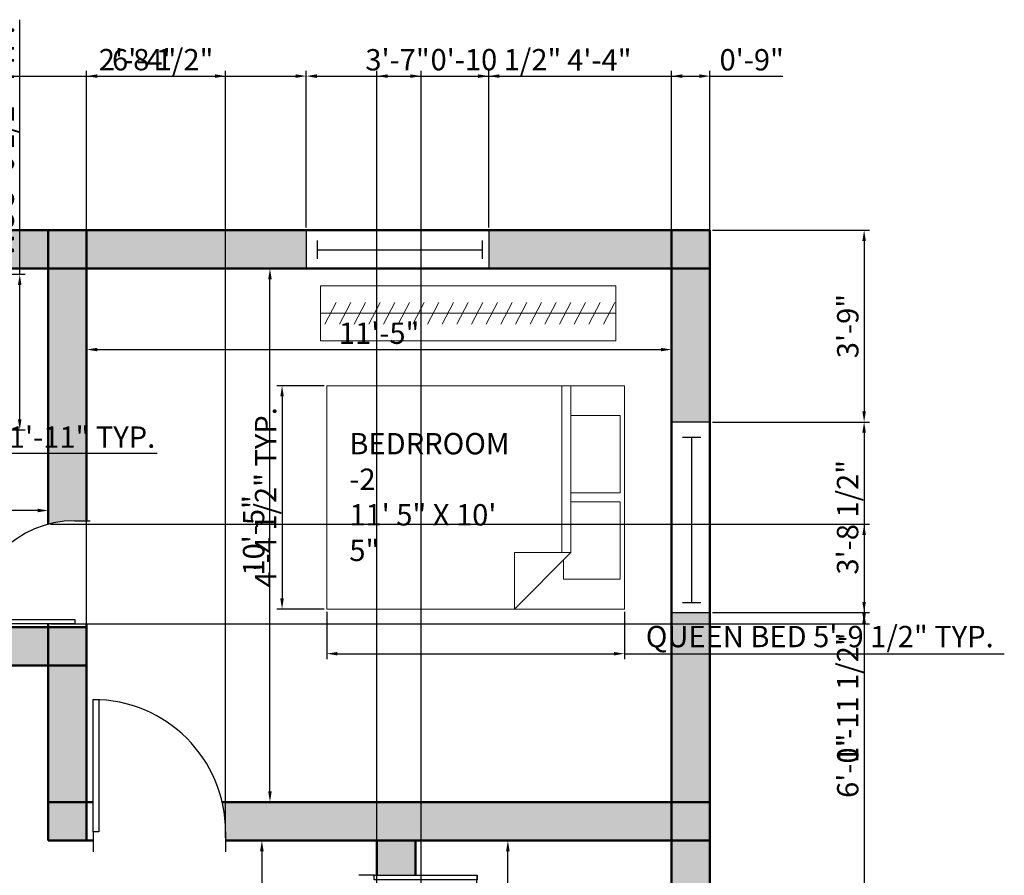
# Model space of a CAD drawing. Units: millimetres. Extents: x 2784 to 3697, y 603 to 1406.
# Tile 7 of 10: x 3013 to 3244, y 1205 to 1406. Entities that reach past the tile are written whole.
import ezdxf

# ---------------------------------------------------------------- set-up
doc = ezdxf.new("R2010")
doc.units = ezdxf.units.MM
for name, color, linetype, lineweight in [('A-ANNO-DIMS', 140, 'Continuous', 18), ('A-AREA-IDEN', 150, 'Continuous', 25), ('A-DOOR', 10, 'Continuous', 25), ('A-FURN', 80, 'Continuous', 18), ('A-GLAZ', 30, 'Continuous', 25), ('A-WALL', 2, 'Continuous', 50), ('A-WALL-PATT', 8, 'Continuous', 13)]:
    doc.layers.add(name, color=color, linetype=linetype, lineweight=lineweight)
doc.styles.get("Standard").update_dxf_attribs({"font": 'arial.ttf'})
doc.dimstyles.new('ISO-25', dxfattribs={"dimtxt": 5, "dimasz": 2.5, "dimexe": 1.25, "dimexo": 0.625, "dimtad": 1, "dimdec": 0, "dimlunit": 3, "dimtxsty": 'Standard', "dimcen": 2.5, "dimadec": 0, "dimazin": 0, "dimtfac": 1, "dimtdec": 0, "dimtmove": 0, "dimatfit": 3, "dimfxl": 1, "dimarcsym": 0})

# ---------------------------------------------------------------- blocks, each defined once
blk = doc.blocks.new('*U2')
for p, q in [((0, 0), (0, -6)), ((40, 0), (40, -6))]:
    blk.add_line(p, q)
blk.add_lwpolyline([(0, 0), (0, 40), (1.75, 40), (1.75, 0)], close=True)
blk.add_arc((0, 0), 40, 0, 90)
blk = doc.blocks.new('*U4')
for p, q in [((0, 4), (0, 0)), ((36, 4), (36, 0)), ((0, 2), (36, 2))]:
    blk.add_line(p, q)
blk = doc.blocks.new('Bed - Queen')
for p, q in [((0, -80.00003), (0, 0)), ((0, 0), (59.99999, 0)), ((59.99999, 0), (59.99999, -80.00003)), ((7.99999, -1.2), (28.79998, -1.2)), ((7.99999, -14.4), (7.99999, -1.2)), ((28.79998, -1.2), (28.79998, -14.4)), ((31.19999, -1.2), (51.99999, -1.2)), ((31.19999, -14.4), (31.19999, -1.2)), ((51.99999, -1.2), (51.99999, -16.4)), ((0, -14.4), (44.8, -14.4)), ((59.99999, -29.6), (44.8, -14.4)), ((44.8, -14.4), (44.8, -29.6)), ((44.8, -16.8), (0, -16.8)), ((51.99999, -16.4), (46.79936, -16.4)), ((44.8, -29.6), (59.99999, -29.6)), ((59.99999, -80.00003), (0, -80.00003))]:
    blk.add_line(p, q)
blk = doc.blocks.new('*D18')
at = {"layer": 'A-ANNO-DIMS', "color": 0, "lineweight": -2, "transparency": 16777216}
for p, q in [((2971.91, 1291.46), (2971.91, 1289.3)), ((3019.91, 1291.46), (3019.91, 1289.3)), ((3017.41, 1290.55), (2974.41, 1290.55))]:
    blk.add_line(p, q, dxfattribs=at)
at = {"layer": 'A-ANNO-DIMS', "color": 0, "transparency": 16777216}
for points in [[(2974.41, 1290.97), (2974.41, 1290.13), (2971.91, 1290.55)], [(3017.41, 1290.97), (3017.41, 1290.13), (3019.91, 1290.55)]]:
    blk.add_solid(points, dxfattribs=at)
at = {"layer": 'Defpoints', "color": 0, "transparency": 16777216}
for p in [(2971.91, 1292.08), (3019.91, 1292.08), (2971.91, 1290.55)]:
    blk.add_point(p, dxfattribs=at)
at = {"layer": 'A-ANNO-DIMS', "color": 0, "transparency": 16777216, "insert": (2995.91, 1293.67), "char_height": 5, "attachment_point": 5}
blk.add_mtext("4'", dxfattribs=at)
blk = doc.blocks.new('*D19')
at = {"layer": 'A-ANNO-DIMS', "color": 0, "lineweight": -2, "transparency": 16777216}
for p, q in [((3072.89, 1347.23), (3070.59, 1347.23)), ((3071.84, 1224.73), (3071.84, 1344.73)), ((3072.89, 1222.23), (3070.59, 1222.23))]:
    blk.add_line(p, q, dxfattribs=at)
at = {"layer": 'A-ANNO-DIMS', "color": 0, "transparency": 16777216}
for points in [[(3071.43, 1344.73), (3072.26, 1344.73), (3071.84, 1347.23)], [(3071.43, 1224.73), (3072.26, 1224.73), (3071.84, 1222.23)]]:
    blk.add_solid(points, dxfattribs=at)
at = {"layer": 'Defpoints', "color": 0, "transparency": 16777216}
for p in [(3071.84, 1347.23), (3073.51, 1347.23), (3073.51, 1222.23)]:
    blk.add_point(p, dxfattribs=at)
at = {"layer": 'A-ANNO-DIMS', "color": 0, "transparency": 16777216, "insert": (3068.66, 1284.73), "char_height": 5, "attachment_point": 5, "rotation": 90}
blk.add_mtext('10\'-5"', dxfattribs=at)
blk = doc.blocks.new('*D20')
at = {"layer": 'A-ANNO-DIMS', "color": 0, "lineweight": -2, "transparency": 16777216}
for p, q in [((3028.91, 1322.82), (3028.91, 1329.51)), ((3165.91, 1328.88), (3165.91, 1329.51)), ((3031.41, 1328.26), (3163.41, 1328.26))]:
    blk.add_line(p, q, dxfattribs=at)
at = {"layer": 'A-ANNO-DIMS', "color": 0, "transparency": 16777216}
for points in [[(3031.41, 1328.67), (3031.41, 1327.84), (3028.91, 1328.26)], [(3163.41, 1328.67), (3163.41, 1327.84), (3165.91, 1328.26)]]:
    blk.add_solid(points, dxfattribs=at)
at = {"layer": 'Defpoints', "color": 0, "transparency": 16777216}
for p in [(3165.91, 1328.26), (3165.91, 1328.26), (3028.91, 1322.19)]:
    blk.add_point(p, dxfattribs=at)
at = {"layer": 'A-ANNO-DIMS', "color": 0, "transparency": 16777216, "insert": (3097.41, 1331.44), "char_height": 5, "attachment_point": 5}
blk.add_mtext('11\'-5"', dxfattribs=at)
blk = doc.blocks.new('*D24')
at = {"layer": 'A-ANNO-DIMS', "color": 0, "lineweight": -2, "transparency": 16777216}
for p, q in [((3124.34, 1213.23), (3128.82, 1213.23)), ((3127.57, 1150.73), (3127.57, 1210.73)), ((3124.34, 1148.23), (3128.82, 1148.23))]:
    blk.add_line(p, q, dxfattribs=at)
at = {"layer": 'A-ANNO-DIMS', "color": 0, "transparency": 16777216}
for points in [[(3127.15, 1210.73), (3127.98, 1210.73), (3127.57, 1213.23)], [(3127.15, 1150.73), (3127.98, 1150.73), (3127.57, 1148.23)]]:
    blk.add_solid(points, dxfattribs=at)
at = {"layer": 'Defpoints', "color": 0, "transparency": 16777216}
for p in [(3123.72, 1213.23), (3127.57, 1213.23), (3123.72, 1148.23)]:
    blk.add_point(p, dxfattribs=at)
at = {"layer": 'A-ANNO-DIMS', "color": 0, "transparency": 16777216, "insert": (3124.4, 1180.73), "char_height": 5, "attachment_point": 5, "rotation": 90}
blk.add_mtext('5\'-5"', dxfattribs=at)
blk = doc.blocks.new('*D37')
at = {"layer": 'A-ANNO-DIMS', "color": 0, "lineweight": -2, "transparency": 16777216}
for p, q in [((3069.6, 1213.23), (3068.7, 1213.23)), ((3069.95, 1210.73), (3069.95, 1081.73)), ((3069.6, 1079.23), (3068.7, 1079.23))]:
    blk.add_line(p, q, dxfattribs=at)
at = {"layer": 'A-ANNO-DIMS', "color": 0, "transparency": 16777216}
for points in [[(3069.53, 1210.73), (3070.37, 1210.73), (3069.95, 1213.23)], [(3069.53, 1081.73), (3070.37, 1081.73), (3069.95, 1079.23)]]:
    blk.add_solid(points, dxfattribs=at)
at = {"layer": 'Defpoints', "color": 0, "transparency": 16777216}
for p in [(3070.22, 1213.23), (3069.95, 1079.23), (3070.22, 1079.23)]:
    blk.add_point(p, dxfattribs=at)
at = {"layer": 'A-ANNO-DIMS', "color": 0, "transparency": 16777216, "insert": (3066.81, 1146.23), "char_height": 5, "attachment_point": 5, "rotation": 90}
blk.add_mtext('11\'-2"', dxfattribs=at)
blk = doc.blocks.new('*D60')
at = {"layer": 'A-ANNO-DIMS', "color": 0, "lineweight": -2, "transparency": 16777216}
for p, q in [((3085.15, 1266.84), (3085.15, 1255.75)), ((3154.89, 1266.84), (3154.89, 1255.75)), ((3087.65, 1257), (3152.39, 1257)), ((3154.89, 1257), (3243.84, 1257))]:
    blk.add_line(p, q, dxfattribs=at)
at = {"layer": 'A-ANNO-DIMS', "color": 0, "transparency": 16777216}
for points in [[(3087.65, 1257.42), (3087.65, 1256.59), (3085.15, 1257)], [(3152.39, 1257.42), (3152.39, 1256.59), (3154.89, 1257)]]:
    blk.add_solid(points, dxfattribs=at)
at = {"layer": 'Defpoints', "color": 0, "transparency": 16777216}
for p in [(3085.15, 1267.47), (3154.89, 1267.47), (3154.89, 1257)]:
    blk.add_point(p, dxfattribs=at)
at = {"layer": 'A-ANNO-DIMS', "color": 0, "transparency": 16777216, "insert": (3200.62, 1260.37), "char_height": 5, "attachment_point": 5}
blk.add_mtext('QUEEN BED 5\'-9 1/2" TYP.', dxfattribs=at)
blk = doc.blocks.new('*D61')
at = {"layer": 'A-ANNO-DIMS', "color": 0, "lineweight": -2, "transparency": 16777216}
for p, q in [((3084.52, 1319.77), (3073.43, 1319.77)), ((3074.68, 1317.27), (3074.68, 1269.97)), ((3084.52, 1267.47), (3073.43, 1267.47))]:
    blk.add_line(p, q, dxfattribs=at)
at = {"layer": 'A-ANNO-DIMS', "color": 0, "transparency": 16777216}
for points in [[(3074.27, 1317.27), (3075.1, 1317.27), (3074.68, 1319.77)], [(3074.27, 1269.97), (3075.1, 1269.97), (3074.68, 1267.47)]]:
    blk.add_solid(points, dxfattribs=at)
at = {"layer": 'Defpoints', "color": 0, "transparency": 16777216}
for p in [(3085.15, 1319.77), (3074.68, 1267.47), (3085.15, 1267.47)]:
    blk.add_point(p, dxfattribs=at)
at = {"layer": 'A-ANNO-DIMS', "color": 0, "transparency": 16777216, "insert": (3071.47, 1293.62), "char_height": 5, "attachment_point": 5, "rotation": 90}
blk.add_mtext('4\'-4 1/2" TYP.', dxfattribs=at)
blk = doc.blocks.new('*D72')
at = {"layer": 'A-ANNO-DIMS', "color": 0, "lineweight": -2, "transparency": 16777216}
for p, q in [((3013.24, 1345.89), (3013.24, 1405.55)), ((3008.39, 1345.89), (3014.49, 1345.89)), ((3013.24, 1311.94), (3013.24, 1343.39)), ((3008.39, 1309.44), (3014.49, 1309.44))]:
    blk.add_line(p, q, dxfattribs=at)
at = {"layer": 'A-ANNO-DIMS', "color": 0, "transparency": 16777216}
for points in [[(3012.82, 1343.39), (3013.65, 1343.39), (3013.24, 1345.89)], [(3012.82, 1311.94), (3013.65, 1311.94), (3013.24, 1309.44)]]:
    blk.add_solid(points, dxfattribs=at)
at = {"layer": 'Defpoints', "color": 0, "transparency": 16777216}
for p in [(3007.77, 1345.89), (3013.24, 1345.89), (3007.77, 1309.44)]:
    blk.add_point(p, dxfattribs=at)
at = {"layer": 'A-ANNO-DIMS', "color": 0, "transparency": 16777216, "insert": (3010.03, 1376.97), "char_height": 5, "attachment_point": 5, "rotation": 90}
blk.add_mtext('WC 3\'-0 1/2" TYP.', dxfattribs=at)
blk = doc.blocks.new('*D73')
at = {"layer": 'A-ANNO-DIMS', "color": 0, "lineweight": -2, "transparency": 16777216}
for p, q in [((2984.6, 1308.81), (2984.6, 1302.72)), ((3007.77, 1308.81), (3007.77, 1302.72)), ((2987.1, 1303.97), (3005.27, 1303.97)), ((3007.77, 1303.97), (3045.41, 1303.97))]:
    blk.add_line(p, q, dxfattribs=at)
at = {"layer": 'A-ANNO-DIMS', "color": 0, "transparency": 16777216}
for points in [[(2987.1, 1304.38), (2987.1, 1303.55), (2984.6, 1303.97)], [(3005.27, 1304.38), (3005.27, 1303.55), (3007.77, 1303.97)]]:
    blk.add_solid(points, dxfattribs=at)
at = {"layer": 'Defpoints', "color": 0, "transparency": 16777216}
for p in [(2984.6, 1309.44), (3007.77, 1309.44), (3007.77, 1303.97)]:
    blk.add_point(p, dxfattribs=at)
at = {"layer": 'A-ANNO-DIMS', "color": 0, "transparency": 16777216, "insert": (3027.84, 1307.1), "char_height": 5, "attachment_point": 5}
blk.add_mtext('1\'-11" TYP.', dxfattribs=at)
blk = doc.blocks.new('*D80')
at = {"layer": 'A-ANNO-DIMS', "color": 0, "lineweight": -2, "transparency": 16777216}
for p, q in [((3004.44, 1356.86), (3004.44, 1393.58)), ((3080.34, 1356.86), (3080.34, 1393.58)), ((3006.94, 1392.33), (3077.84, 1392.33))]:
    blk.add_line(p, q, dxfattribs=at)
at = {"layer": 'A-ANNO-DIMS', "color": 0, "transparency": 16777216}
for points in [[(3006.94, 1392.75), (3006.94, 1391.91), (3004.44, 1392.33)], [(3077.84, 1392.75), (3077.84, 1391.91), (3080.34, 1392.33)]]:
    blk.add_solid(points, dxfattribs=at)
at = {"layer": 'Defpoints', "color": 0, "transparency": 16777216}
for p in [(3080.34, 1392.33), (3004.44, 1356.23), (3080.34, 1356.23)]:
    blk.add_point(p, dxfattribs=at)
at = {"layer": 'A-ANNO-DIMS', "color": 0, "transparency": 16777216, "insert": (3042.39, 1395.51), "char_height": 5, "attachment_point": 5}
blk.add_mtext('6\'-4"', dxfattribs=at)
blk = doc.blocks.new('*D81')
at = {"layer": 'A-ANNO-DIMS', "color": 0, "lineweight": -2, "transparency": 16777216}
for p, q in [((3080.34, 1356.86), (3080.34, 1393.58)), ((3123.1, 1356.86), (3123.1, 1393.58)), ((3082.84, 1392.33), (3120.6, 1392.33))]:
    blk.add_line(p, q, dxfattribs=at)
at = {"layer": 'A-ANNO-DIMS', "color": 0, "transparency": 16777216}
for points in [[(3082.84, 1392.75), (3082.84, 1391.91), (3080.34, 1392.33)], [(3120.6, 1392.75), (3120.6, 1391.91), (3123.1, 1392.33)]]:
    blk.add_solid(points, dxfattribs=at)
at = {"layer": 'Defpoints', "color": 0, "transparency": 16777216}
for p in [(3123.1, 1392.33), (3080.34, 1356.23), (3123.1, 1356.23)]:
    blk.add_point(p, dxfattribs=at)
at = {"layer": 'A-ANNO-DIMS', "color": 0, "transparency": 16777216, "insert": (3101.72, 1395.51), "char_height": 5, "attachment_point": 5}
blk.add_mtext('3\'-7"', dxfattribs=at)
blk = doc.blocks.new('*D82')
at = {"layer": 'A-ANNO-DIMS', "color": 0, "lineweight": -2, "transparency": 16777216}
for p, q in [((3123.1, 1356.86), (3123.1, 1393.58)), ((3174.91, 1356.86), (3174.91, 1393.58)), ((3125.6, 1392.33), (3172.41, 1392.33))]:
    blk.add_line(p, q, dxfattribs=at)
at = {"layer": 'A-ANNO-DIMS', "color": 0, "transparency": 16777216}
for points in [[(3125.6, 1392.75), (3125.6, 1391.91), (3123.1, 1392.33)], [(3172.41, 1392.75), (3172.41, 1391.91), (3174.91, 1392.33)]]:
    blk.add_solid(points, dxfattribs=at)
at = {"layer": 'Defpoints', "color": 0, "transparency": 16777216}
for p in [(3174.91, 1392.33), (3123.1, 1356.23), (3174.91, 1356.23)]:
    blk.add_point(p, dxfattribs=at)
at = {"layer": 'A-ANNO-DIMS', "color": 0, "transparency": 16777216, "insert": (3149, 1395.46), "char_height": 5, "attachment_point": 5}
blk.add_mtext('4\'-4"', dxfattribs=at)
blk = doc.blocks.new('*D91')
at = {"layer": 'A-ANNO-DIMS', "color": 0, "lineweight": -2, "transparency": 16777216}
for p, q in [((3175.53, 1356.23), (3212.26, 1356.23)), ((3211.01, 1353.73), (3211.01, 1313.78)), ((3175.53, 1311.28), (3212.26, 1311.28))]:
    blk.add_line(p, q, dxfattribs=at)
at = {"layer": 'A-ANNO-DIMS', "color": 0, "transparency": 16777216}
for points in [[(3210.59, 1353.73), (3211.42, 1353.73), (3211.01, 1356.23)], [(3210.59, 1313.78), (3211.42, 1313.78), (3211.01, 1311.28)]]:
    blk.add_solid(points, dxfattribs=at)
at = {"layer": 'Defpoints', "color": 0, "transparency": 16777216}
for p in [(3174.91, 1356.23), (3174.91, 1311.28), (3211.01, 1311.28)]:
    blk.add_point(p, dxfattribs=at)
at = {"layer": 'A-ANNO-DIMS', "color": 0, "transparency": 16777216, "insert": (3207.83, 1333.76), "char_height": 5, "attachment_point": 5, "rotation": 90}
blk.add_mtext('3\'-9"', dxfattribs=at)
blk = doc.blocks.new('*D92')
at = {"layer": 'A-ANNO-DIMS', "color": 0, "lineweight": -2, "transparency": 16777216}
for p, q in [((3175.53, 1311.28), (3212.26, 1311.28)), ((3211.01, 1308.78), (3211.01, 1269.15)), ((3175.53, 1266.65), (3212.26, 1266.65))]:
    blk.add_line(p, q, dxfattribs=at)
at = {"layer": 'A-ANNO-DIMS', "color": 0, "transparency": 16777216}
for points in [[(3210.59, 1308.78), (3211.42, 1308.78), (3211.01, 1311.28)], [(3210.59, 1269.15), (3211.42, 1269.15), (3211.01, 1266.65)]]:
    blk.add_solid(points, dxfattribs=at)
at = {"layer": 'Defpoints', "color": 0, "transparency": 16777216}
for p in [(3174.91, 1311.28), (3174.91, 1266.65), (3211.01, 1266.65)]:
    blk.add_point(p, dxfattribs=at)
at = {"layer": 'A-ANNO-DIMS', "color": 0, "transparency": 16777216, "insert": (3207.79, 1288.96), "char_height": 5, "attachment_point": 5, "rotation": 90}
blk.add_mtext('3\'-8 1/2"', dxfattribs=at)
blk = doc.blocks.new('*D93')
at = {"layer": 'A-ANNO-DIMS', "color": 0, "lineweight": -2, "transparency": 16777216}
for p, q in [((3175.53, 1266.65), (3212.26, 1266.65)), ((3211.01, 1264.15), (3211.01, 1197.33)), ((3175.53, 1194.83), (3212.26, 1194.83))]:
    blk.add_line(p, q, dxfattribs=at)
at = {"layer": 'A-ANNO-DIMS', "color": 0, "transparency": 16777216}
for points in [[(3210.59, 1264.15), (3211.42, 1264.15), (3211.01, 1266.65)], [(3210.59, 1197.33), (3211.42, 1197.33), (3211.01, 1194.83)]]:
    blk.add_solid(points, dxfattribs=at)
at = {"layer": 'Defpoints', "color": 0, "transparency": 16777216}
for p in [(3174.91, 1266.65), (3174.91, 1194.83), (3211.01, 1194.83)]:
    blk.add_point(p, dxfattribs=at)
at = {"layer": 'A-ANNO-DIMS', "color": 0, "transparency": 16777216, "insert": (3207.83, 1230.74), "char_height": 5, "attachment_point": 5, "rotation": 90}
blk.add_mtext('6\'-0"', dxfattribs=at)
blk = doc.blocks.new('*D101')
at = {"layer": 'A-ANNO-DIMS', "color": 0, "lineweight": -2, "transparency": 16777216}
for p, q in [((3028.91, 1213.86), (3028.91, 1393.58)), ((3061.45, 1213.86), (3061.45, 1393.58)), ((3031.41, 1392.33), (3058.95, 1392.33))]:
    blk.add_line(p, q, dxfattribs=at)
at = {"layer": 'A-ANNO-DIMS', "color": 0, "transparency": 16777216}
for points in [[(3031.41, 1392.75), (3031.41, 1391.91), (3028.91, 1392.33)], [(3058.95, 1392.75), (3058.95, 1391.91), (3061.45, 1392.33)]]:
    blk.add_solid(points, dxfattribs=at)
at = {"layer": 'Defpoints', "color": 0, "transparency": 16777216}
for p in [(3061.45, 1392.33), (3028.91, 1213.23), (3061.45, 1213.23)]:
    blk.add_point(p, dxfattribs=at)
at = {"layer": 'A-ANNO-DIMS', "color": 0, "transparency": 16777216, "insert": (3045.18, 1395.54), "char_height": 5, "attachment_point": 5}
blk.add_mtext('2\'-8 1/2"', dxfattribs=at)
blk = doc.blocks.new('*D105')
at = {"layer": 'A-ANNO-DIMS', "color": 0, "lineweight": -2, "transparency": 16777216}
for p, q in [((3020.44, 1287.32), (3212.26, 1287.32)), ((3211.01, 1284.82), (3211.01, 1266.49)), ((3020.53, 1263.99), (3212.26, 1263.99)), ((3211.01, 1263.99), (3211.01, 1231.89))]:
    blk.add_line(p, q, dxfattribs=at)
at = {"layer": 'A-ANNO-DIMS', "color": 0, "transparency": 16777216}
for points in [[(3210.59, 1284.82), (3211.42, 1284.82), (3211.01, 1287.32)], [(3210.59, 1266.49), (3211.42, 1266.49), (3211.01, 1263.99)]]:
    blk.add_solid(points, dxfattribs=at)
at = {"layer": 'Defpoints', "color": 0, "transparency": 16777216}
for p in [(3019.81, 1287.32), (3019.91, 1263.99), (3211.01, 1263.99)]:
    blk.add_point(p, dxfattribs=at)
at = {"layer": 'A-ANNO-DIMS', "color": 0, "transparency": 16777216, "insert": (3207.8, 1246.69), "char_height": 5, "attachment_point": 5, "rotation": 90}
blk.add_mtext('1\'-11 1/2"', dxfattribs=at)
blk = doc.blocks.new('*D108')
at = {"layer": 'A-ANNO-DIMS', "color": 0, "lineweight": -2, "transparency": 16777216}
for p, q in [((3165.91, 1169.69), (3165.91, 1393.58)), ((3174.91, 1169.69), (3174.91, 1393.58)), ((3168.41, 1392.33), (3172.41, 1392.33)), ((3174.91, 1392.33), (3191.95, 1392.33))]:
    blk.add_line(p, q, dxfattribs=at)
at = {"layer": 'A-ANNO-DIMS', "color": 0, "transparency": 16777216}
for points in [[(3168.41, 1392.75), (3168.41, 1391.91), (3165.91, 1392.33)], [(3172.41, 1392.75), (3172.41, 1391.91), (3174.91, 1392.33)]]:
    blk.add_solid(points, dxfattribs=at)
at = {"layer": 'Defpoints', "color": 0, "transparency": 16777216}
for p in [(3174.91, 1392.33), (3165.91, 1169.06), (3174.91, 1169.06)]:
    blk.add_point(p, dxfattribs=at)
at = {"layer": 'A-ANNO-DIMS', "color": 0, "transparency": 16777216, "insert": (3184.68, 1395.51), "char_height": 5, "attachment_point": 5}
blk.add_mtext('0\'-9"', dxfattribs=at)
blk = doc.blocks.new('*D109')
at = {"layer": 'A-ANNO-DIMS', "color": 0, "lineweight": -2, "transparency": 16777216}
for p, q in [((3096.91, 1139.86), (3096.91, 1393.58)), ((3107.23, 1133.86), (3107.23, 1393.58)), ((3099.41, 1392.33), (3104.73, 1392.33)), ((3107.23, 1392.33), (3139.81, 1392.33))]:
    blk.add_line(p, q, dxfattribs=at)
at = {"layer": 'A-ANNO-DIMS', "color": 0, "transparency": 16777216}
for points in [[(3099.41, 1392.75), (3099.41, 1391.91), (3096.91, 1392.33)], [(3104.73, 1392.75), (3104.73, 1391.91), (3107.23, 1392.33)]]:
    blk.add_solid(points, dxfattribs=at)
at = {"layer": 'Defpoints', "color": 0, "transparency": 16777216}
for p in [(3107.23, 1392.33), (3096.91, 1139.23), (3107.23, 1133.24)]:
    blk.add_point(p, dxfattribs=at)
at = {"layer": 'A-ANNO-DIMS', "color": 0, "transparency": 16777216, "insert": (3124.77, 1395.54), "char_height": 5, "attachment_point": 5}
blk.add_mtext('0\'-10 1/2"', dxfattribs=at)

msp = doc.modelspace()

# ---------------------------------------------------------------- hatches: boundary and pattern name
at = {"layer": 'A-WALL-PATT'}
h = msp.add_hatch(color=256, dxfattribs=at)
h.dxf.hatch_style = 1
h.paths.add_polyline_path([(2869.53, 1356.23), (2839.91, 1356.23), (2839.91, 1347.23), (2869.53, 1347.23)])
h.paths.add_polyline_path([(2839.91, 1356.23), (2830.91, 1356.23), (2830.91, 1347.23), (2839.91, 1347.23)])
h.paths.add_polyline_path([(2839.91, 1347.23), (2830.91, 1347.23), (2830.91, 1314.23), (2839.91, 1314.23)])
h.paths.add_polyline_path([(2839.91, 1268.19), (2830.91, 1268.19), (2830.91, 1222.23), (2839.91, 1222.23)])
h.paths.add_polyline_path([(2839.91, 1222.23), (2830.91, 1222.23), (2830.91, 1213.23), (2839.91, 1213.23)])
h.paths.add_polyline_path([(2962.91, 1222.23), (2839.91, 1222.23), (2839.91, 1213.23), (2962.91, 1213.23)])
h.paths.add_polyline_path([(2971.91, 1222.23), (2962.91, 1222.23), (2962.91, 1213.23), (2971.91, 1213.23)])
h.paths.add_polyline_path([(2971.91, 1263.23), (2962.91, 1263.23), (2962.91, 1254.23), (2971.91, 1254.23)])
h.paths.add_polyline_path([(2971.91, 1347.23), (2962.91, 1347.23), (2962.91, 1263.23), (2971.91, 1263.23)])
h.paths.add_polyline_path([(2971.91, 1356.23), (2962.91, 1356.23), (2962.91, 1347.23), (2971.91, 1347.23)])
h.paths.add_polyline_path([(2962.91, 1356.23), (2913.7, 1356.23), (2913.7, 1347.23), (2962.91, 1347.23)])
h.paths.add_polyline_path([(2982.62, 1356.23), (2971.91, 1356.23), (2971.91, 1347.23), (2982.62, 1347.23)])
h.paths.add_polyline_path([(3019.91, 1356.23), (3004.44, 1356.23), (3004.44, 1347.23), (3019.91, 1347.23)])
h.paths.add_polyline_path([(3028.91, 1356.23), (3019.91, 1356.23), (3019.91, 1347.23), (3028.91, 1347.23)])
h.paths.add_polyline_path([(3028.91, 1347.23), (3019.91, 1347.23), (3019.91, 1287.35, -0.06506), (3026.12, 1288.16), (3028.91, 1288.16)])
h.paths.add_polyline_path([(3019.91, 1263.23), (2971.91, 1263.23), (2971.91, 1254.23), (3019.91, 1254.23)])
h.paths.add_polyline_path([(3028.91, 1263.23), (3019.91, 1263.23), (3019.91, 1254.23), (3028.91, 1254.23)])
h.paths.add_polyline_path([(3028.91, 1254.23), (3019.91, 1254.23), (3019.91, 1222.23), (3028.91, 1222.23)])
h.paths.add_polyline_path([(3028.91, 1222.23), (3019.91, 1222.23), (3019.91, 1213.23), (3028.91, 1213.23)])
h.paths.add_polyline_path([(3165.91, 1222.23), (3060.65, 1222.23, -0.056956), (3061.45, 1215.23), (3061.45, 1213.23), (3165.91, 1213.23)])
h.paths.add_polyline_path([(3080.34, 1356.23), (3028.91, 1356.23), (3028.91, 1347.23), (3080.34, 1347.23)])
h.paths.add_polyline_path([(3174.91, 1347.23), (3165.91, 1347.23), (3165.91, 1311.28), (3174.91, 1311.28)])
h.paths.add_polyline_path([(3174.91, 1356.23), (3165.91, 1356.23), (3165.91, 1347.23), (3174.91, 1347.23)])
h.paths.add_polyline_path([(3165.91, 1356.23), (3123.1, 1356.23), (3123.1, 1347.23), (3165.91, 1347.23)])
h.paths.add_polyline_path([(3174.91, 1266.65), (3165.91, 1266.65), (3165.91, 1222.23), (3174.91, 1222.23)])
h.paths.add_polyline_path([(3174.91, 1222.23), (3165.91, 1222.23), (3165.91, 1213.23), (3174.91, 1213.23)])
h.paths.add_polyline_path([(3174.91, 1213.23), (3165.91, 1213.23), (3165.91, 1194.83), (3174.91, 1194.83)])
h.paths.add_polyline_path([(3105.91, 1182.92, -0.096276), (3096.91, 1180.92), (3096.91, 1148.23), (3105.91, 1148.23)])
h.paths.add_polyline_path([(3105.91, 1213.23), (3096.91, 1213.23), (3096.91, 1205.07), (3105.91, 1205.07)])
h.paths.add_polyline_path([(2971.91, 1213.23), (2962.91, 1213.23), (2962.91, 1161.09), (2971.91, 1161.09)])
h.paths.add_polyline_path([(2839.91, 1213.23), (2830.91, 1213.23), (2830.91, 1157.46), (2839.91, 1157.46)])
h.paths.add_polyline_path([(2839.91, 1108.88), (2830.91, 1108.88), (2830.91, 1042.23), (2839.91, 1042.23)])
h.paths.add_polyline_path([(2839.91, 1042.23), (2830.91, 1042.23), (2830.91, 1033.23), (2839.91, 1033.23)])
h.paths.add_polyline_path([(2881.91, 1042.23), (2839.91, 1042.23), (2839.91, 1033.23), (2881.91, 1033.23)])
h.paths.add_polyline_path([(2996.91, 1042.23), (2890.91, 1042.23), (2890.91, 1033.23), (2996.91, 1033.23)])
h.paths.add_polyline_path([(2890.91, 1042.23), (2881.91, 1042.23), (2881.91, 1033.23), (2890.91, 1033.23)])
h.paths.add_polyline_path([(2890.91, 1033.23), (2881.91, 1033.23), (2881.91, 984.23), (2890.91, 984.23)])
h.paths.add_polyline_path([(2839.91, 1033.23), (2830.91, 1033.23), (2830.91, 984.23), (2839.91, 984.23)])
h.paths.add_polyline_path([(2839.91, 984.23), (2830.91, 984.23), (2830.91, 975.23), (2839.91, 975.23)])
h.paths.add_polyline_path([(2881.91, 984.23), (2854.14, 984.23, -0.154991), (2857.05, 975.23), (2881.91, 975.23)])
h.paths.add_polyline_path([(2890.91, 984.23), (2881.91, 984.23), (2881.91, 975.23), (2890.91, 975.23)])
h.paths.add_polyline_path([(2900.85, 984.23), (2890.91, 984.23), (2890.91, 975.23), (2900.85, 975.23), (2900.85, 975.78)])
h.paths.add_polyline_path([(2996.91, 984.23), (2923.49, 984.23, -0.089525), (2925.01, 975.78), (2925.01, 975.23), (2996.91, 975.23)])
h.paths.add_polyline_path([(3165.91, 984.23), (3005.91, 984.23), (3005.91, 975.23), (3165.91, 975.23)])
h.paths.add_polyline_path([(3005.91, 1033.23), (2996.91, 1033.23), (2996.91, 984.23), (3005.91, 984.23)])
h.paths.add_polyline_path([(3005.91, 984.23), (2996.91, 984.23), (2996.91, 975.23), (3005.91, 975.23)])
h.paths.add_polyline_path([(3005.91, 1042.23), (2996.91, 1042.23), (2996.91, 1033.23), (3005.91, 1033.23)])
h.paths.add_polyline_path([(3096.91, 1079.23), (2971.91, 1079.23), (2971.91, 1070.23), (3096.91, 1070.23)])
h.paths.add_polyline_path([(2971.91, 1079.23), (2962.91, 1079.23), (2962.91, 1070.23), (2971.91, 1070.23)])
h.paths.add_polyline_path([(2971.91, 1070.23), (2962.91, 1070.23), (2962.91, 1060.28, -0.115005), (2971.91, 1066.55)])
h.paths.add_polyline_path([(2971.91, 1105.54), (2962.91, 1105.54), (2962.91, 1079.23), (2971.91, 1079.23)])
h.paths.add_polyline_path([(3165.91, 1079.23), (3105.91, 1079.23), (3105.91, 1070.23), (3165.91, 1070.23)])
h.paths.add_polyline_path([(3105.91, 1079.23), (3096.91, 1079.23), (3096.91, 1070.23), (3105.91, 1070.23)])
h.paths.add_polyline_path([(3105.91, 1148.23), (3096.91, 1148.23), (3096.91, 1139.23), (3105.91, 1139.23)])
h.paths.add_polyline_path([(3105.91, 1139.23), (3096.91, 1139.23), (3096.91, 1104.7), (3098.08, 1104.75, -0.08216), (3105.91, 1103.81)])
h.paths.add_polyline_path([(3165.91, 1148.23), (3105.91, 1148.23), (3105.91, 1139.23), (3165.91, 1139.23)])
h.paths.add_polyline_path([(3174.91, 1148.23), (3165.91, 1148.23), (3165.91, 1139.23), (3174.91, 1139.23)])
h.paths.add_polyline_path([(3174.91, 1139.23), (3165.91, 1139.23), (3165.91, 1123.86), (3174.91, 1123.86)])
h.paths.add_polyline_path([(3174.91, 1097.37), (3165.91, 1097.37), (3165.91, 1079.23), (3174.91, 1079.23)])
h.paths.add_polyline_path([(3174.91, 1079.23), (3165.91, 1079.23), (3165.91, 1070.23), (3174.91, 1070.23)])
h.paths.add_polyline_path([(3174.91, 1070.23), (3165.91, 1070.23), (3165.91, 1048.77), (3174.91, 1048.77)])
h.paths.add_polyline_path([(3174.91, 1002.74), (3165.91, 1002.74), (3165.91, 984.23), (3174.91, 984.23)])
h.paths.add_polyline_path([(3174.91, 984.23), (3165.91, 984.23), (3165.91, 975.23), (3174.91, 975.23)])
h.paths.add_polyline_path([(3174.91, 975.23), (3165.91, 975.23), (3165.91, 725.23), (3174.91, 725.23)])
h.paths.add_polyline_path([(2839.91, 975.23), (2830.91, 975.23), (2830.91, 725.23), (2839.91, 725.23)])
h.paths.add_polyline_path([(3165.91, 725.23), (2839.91, 725.23), (2839.91, 716.23), (3165.91, 716.23)])
h.paths.add_polyline_path([(3174.91, 725.23), (3165.91, 725.23), (3165.91, 716.23), (3174.91, 716.23)])
h.paths.add_polyline_path([(2839.91, 725.23), (2830.91, 725.23), (2830.91, 716.23), (2839.91, 716.23)])

# ---------------------------------------------------------------- linework, layer by layer
at = {"layer": 'A-FURN'}
for p, q in [((3087.32, 1339.3), (3084.67, 1334.22)), ((3090.75, 1339.3), (3088.11, 1334.22)), ((3094.19, 1339.3), (3091.54, 1334.22)), ((3097.63, 1339.3), (3094.98, 1334.22)), ((3101.06, 1339.3), (3098.42, 1334.22)), ((3104.5, 1339.3), (3101.85, 1334.22)), ((3107.94, 1339.3), (3105.29, 1334.22)), ((3111.37, 1339.3), (3108.73, 1334.22)), ((3114.81, 1339.3), (3112.16, 1334.22)), ((3118.25, 1339.3), (3115.6, 1334.22)), ((3121.68, 1339.3), (3119.03, 1334.22)), ((3125.12, 1339.3), (3122.47, 1334.22)), ((3128.56, 1339.3), (3125.91, 1334.22)), ((3131.99, 1339.3), (3129.34, 1334.22)), ((3135.43, 1339.3), (3132.78, 1334.22)), ((3138.87, 1339.3), (3136.22, 1334.22)), ((3142.3, 1339.3), (3139.65, 1334.22)), ((3145.74, 1339.3), (3143.09, 1334.22)), ((3149.18, 1339.3), (3146.53, 1334.22)), ((3152.61, 1339.3), (3149.96, 1334.22)), ((3083.68, 1336.76), (3152.83, 1336.76))]:
    msp.add_line(p, q, dxfattribs=at)
msp.add_lwpolyline([(3152.83, 1343.22), (3083.68, 1343.22), (3083.68, 1330.3), (3152.83, 1330.3)], close=True, dxfattribs=at)
at = {"layer": 'A-GLAZ'}
for p, q in [((3080.34, 1356.23), (3080.34, 1347.23)), ((3123.1, 1356.23), (3123.1, 1347.23)), ((3174.91, 1311.28), (3165.91, 1311.28)), ((3165.91, 1266.65), (3174.91, 1266.65))]:
    msp.add_line(p, q, dxfattribs=at)
at = {"layer": 'A-WALL'}
for p, q in [((2830.91, 1356.23), (3174.91, 1356.23)), ((3019.91, 1356.23), (3019.91, 1287.35)), ((3028.91, 1356.23), (3028.91, 1288.16)), ((3165.91, 1356.23), (3165.91, 1213.23)), ((3174.91, 1356.23), (3174.91, 1213.23)), ((2830.91, 1347.23), (3174.91, 1347.23)), ((3019.91, 1263.99), (3019.91, 1213.23)), ((3028.91, 1263.99), (3028.91, 1213.23)), ((2962.91, 1263.23), (3028.91, 1263.23)), ((2962.91, 1254.23), (3028.91, 1254.23)), ((3019.91, 1222.23), (3030.41, 1222.23)), ((3060.65, 1222.23), (3174.91, 1222.23)), ((3019.91, 1213.23), (3030.41, 1213.23)), ((3061.45, 1213.23), (3174.91, 1213.23)), ((3096.91, 1213.23), (3096.91, 1205.07)), ((3105.91, 1213.23), (3105.91, 1205.07)), ((3165.91, 1213.23), (3165.91, 643.6)), ((3174.91, 1213.23), (3174.91, 643.6))]:
    msp.add_line(p, q, dxfattribs=at)

# ---------------------------------------------------------------- block references
at = {"layer": 'A-DOOR', "xscale": 0.6041131756153701, "yscale": 0.6041131756153701, "zscale": 0.6041131756153701}
for p, rotation in [((3026.12, 1263.99), 90), ((3096.25, 1205.07), 270)]:
    msp.add_blockref('*U2', p, dxfattribs=dict(at, rotation=rotation))
at = {"layer": 'A-DOOR', "xscale": 0.7759495368129277, "yscale": 0.7759495368129277, "zscale": 0.7759495368129277}
msp.add_blockref('*U2', (3030.41, 1215.23), dxfattribs=at)
at = {"layer": 'A-FURN', "xscale": 0.8718255544036225, "yscale": 0.8718255544036225, "zscale": 0.8718255544036225, "rotation": 270}
msp.add_blockref('Bed - Queen', (3154.89, 1319.77), dxfattribs=at)
at = {"layer": 'A-GLAZ', "xscale": 1.074021802203067, "yscale": 1.074021802203067, "zscale": 1.074021802203067}
msp.add_blockref('*U4', (3082.88, 1349.5), dxfattribs=at)
at = {"layer": 'A-GLAZ', "xscale": 1.074021802203067, "yscale": 1.074021802203067, "zscale": 1.074021802203067, "rotation": 270}
msp.add_blockref('*U4', (3168.44, 1307.62), dxfattribs=at)

# ---------------------------------------------------------------- texts
at = {"layer": 'A-AREA-IDEN', "insert": (3090.44, 1308.71), "char_height": 5, "attachment_point": 1}
msp.add_mtext_dynamic_manual_height_columns('BEDRROOM -2 \\P11\' 5" X 10\' 5"', width=36.959, gutter_width=12.5, heights=[0], dxfattribs=at)

# ---------------------------------------------------------------- dimensions: what is measured, and where the dimension line sits
at = {"layer": 'A-ANNO-DIMS'}
for base, p1, p2, angle, text, picture, middle in [((3013.2382, 1345.8915), (3007.7698, 1309.4352), (3007.7698, 1345.8915), 90, 'WC <> TYP.', '*D72', (3010.0262, 1376.9718)), ((3074.68, 1267.47), (3085.15, 1319.77), (3085.15, 1267.47), 270, '<> TYP.', '*D61', (3071.47, 1293.62))]:
    dim = msp.add_linear_dim(base=base, p1=p1, p2=p2, angle=angle, text=text, dimstyle='ISO-25', override={"dimdec": 1, "dimrnd": 0, "dimzin": 1, "dimlunit": 4, "dimfrac": 2}, dxfattribs=at)
    dim.commit()
    dim.dimension.update_dxf_attribs({"geometry": picture, "text_midpoint": middle})
for base, p1, p2, override, picture, middle in [((3061.45, 1392.33), (3028.91, 1213.23), (3061.45, 1213.23), {"dimdec": 1, "dimlfac": 1, "dimrnd": 0, "dimzin": 1, "dimdsep": 46, "dimlunit": 4, "dimfrac": 2}, '*D101', (3045.18, 1395.54)), ((3107.23, 1392.33), (3096.91, 1139.23), (3107.23, 1133.24), {"dimdec": 1, "dimlfac": 1, "dimrnd": 0, "dimzin": 1, "dimdsep": 46, "dimlunit": 4, "dimfrac": 2}, '*D109', (3124.77, 1395.54)), ((3080.34, 1392.33), (3004.44, 1356.23), (3080.34, 1356.23), {"dimdec": 1, "dimlfac": 1, "dimrnd": 0, "dimzin": 1, "dimdsep": 46, "dimlunit": 4, "dimfrac": 2}, '*D80', (3042.39, 1395.51)), ((3123.1, 1392.33), (3080.34, 1356.23), (3123.1, 1356.23), {"dimdec": 1, "dimlfac": 1, "dimrnd": 0, "dimzin": 1, "dimdsep": 46, "dimlunit": 4, "dimfrac": 2}, '*D81', (3101.72, 1395.51)), ((3174.91, 1392.33), (3123.1, 1356.23), (3174.91, 1356.23), {"dimdec": 1, "dimlfac": 1, "dimrnd": 0, "dimzin": 1, "dimdsep": 46, "dimlunit": 4, "dimfrac": 2}, '*D82', (3149, 1395.46)), ((3174.91, 1392.33), (3165.91, 1169.06), (3174.91, 1169.06), {"dimdec": 1, "dimlfac": 1, "dimrnd": 0, "dimzin": 1, "dimdsep": 46, "dimlunit": 4, "dimfrac": 2}, '*D108', (3184.68, 1395.51)), ((3165.91, 1328.26), (3028.91, 1322.19), (3165.91, 1328.26), {"dimclrd": 0, "dimclre": 0, "dimclrt": 0}, '*D20', (3097.41, 1331.44)), ((2971.91, 1290.55), (3019.91, 1292.08), (2971.91, 1292.08), {"dimclrd": 0, "dimclre": 0, "dimclrt": 0}, '*D18', (2995.91, 1293.67))]:
    dim = msp.add_linear_dim(base=base, p1=p1, p2=p2, dimstyle='ISO-25', override=override, dxfattribs=at)
    dim.commit()
    dim.dimension.update_dxf_attribs({"geometry": picture, "text_midpoint": middle})
for base, p1, p2, override, picture, middle in [((3211.0063, 1311.2825), (3174.9063, 1356.231), (3174.9063, 1311.2825), {"dimdec": 1, "dimlfac": 1, "dimrnd": 0, "dimzin": 1, "dimdsep": 46, "dimlunit": 4, "dimfrac": 2}, '*D91', (3207.8268, 1333.7567)), ((3071.84, 1347.23), (3073.51, 1222.23), (3073.51, 1347.23), {"dimclrd": 0, "dimclre": 0, "dimclrt": 0}, '*D19', (3068.66, 1284.73)), ((3211.01, 1266.65), (3174.91, 1311.28), (3174.91, 1266.65), {"dimdec": 1, "dimlfac": 1, "dimrnd": 0, "dimzin": 1, "dimdsep": 46, "dimlunit": 4, "dimfrac": 2}, '*D92', (3207.79, 1288.96)), ((3211.01, 1263.99), (3019.81, 1287.32), (3019.91, 1263.99), {"dimdec": 1, "dimlfac": 1, "dimrnd": 0, "dimzin": 1, "dimdsep": 46, "dimlunit": 4, "dimfrac": 2}, '*D105', (3207.8, 1246.69)), ((3211.01, 1194.83), (3174.91, 1266.65), (3174.91, 1194.83), {"dimdec": 1, "dimlfac": 1, "dimrnd": 0, "dimzin": 1, "dimdsep": 46, "dimlunit": 4, "dimfrac": 2}, '*D93', (3207.83, 1230.74)), ((3069.95, 1079.23), (3070.22, 1213.23), (3070.22, 1079.23), {"dimclrd": 0, "dimclre": 0, "dimclrt": 0}, '*D37', (3066.81, 1146.23)), ((3127.57, 1213.23), (3123.72, 1148.23), (3123.72, 1213.23), {"dimclrd": 0, "dimclre": 0, "dimclrt": 0}, '*D24', (3124.4, 1180.73))]:
    dim = msp.add_linear_dim(base=base, p1=p1, p2=p2, angle=90, dimstyle='ISO-25', override=override, dxfattribs=at)
    dim.commit()
    dim.dimension.update_dxf_attribs({"geometry": picture, "text_midpoint": middle})
for base, p1, p2, text, picture, middle in [((3007.77, 1303.97), (2984.6, 1309.44), (3007.77, 1309.44), '<> TYP.', '*D73', (3027.84, 1307.1)), ((3154.89, 1257), (3085.15, 1267.47), (3154.89, 1267.47), 'QUEEN BED <> TYP.', '*D60', (3200.62, 1260.37))]:
    dim = msp.add_linear_dim(base=base, p1=p1, p2=p2, text=text, dimstyle='ISO-25', override={"dimdec": 1, "dimrnd": 0, "dimzin": 1, "dimlunit": 4, "dimfrac": 2}, dxfattribs=at)
    dim.commit()
    dim.dimension.update_dxf_attribs({"geometry": picture, "text_midpoint": middle})

doc.saveas('drawing.dxf')
